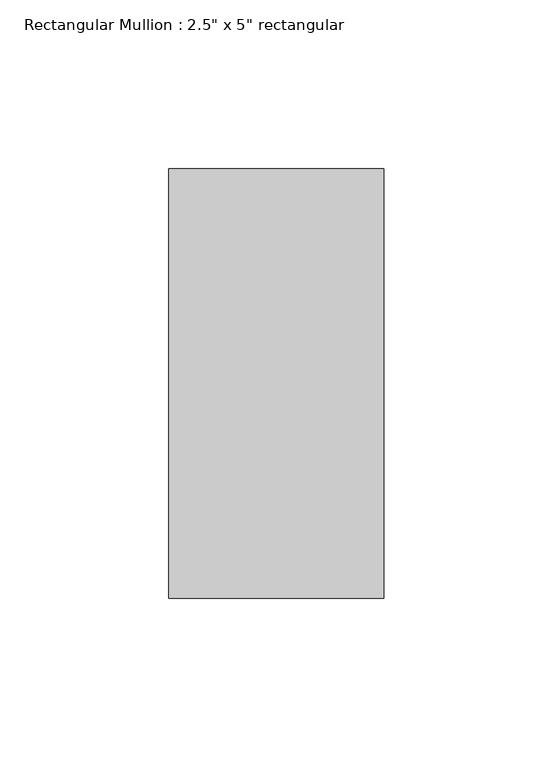
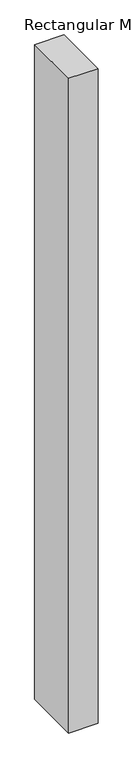
"""IFC4 building model written with IfcOpenShell, lengths in millimetres: member geometry."""

from ifc_helpers import new_model, si_unit, frame, origin, place, context, project, spatial, polyline, outline, extrude, source, transform, mapped, element, save


def member_177cc448(model_context):
    return source(origin(), model_context, "Body", "SweptSolid", [
        extrude(outline(polyline([(0.0, 63.5), (0.0, -63.5), (-63.5, -63.5), (-63.5, 63.5), (0.0, 63.5)])), frame((0.0, 0.0, -1493.5474484), z_axis=(0.0, 0.0, 1.0), x_axis=(1.0, 0.0, 0.0)), (0.0, 0.0, 1.0), 1493.5474484),
    ])


if __name__ == "__main__":
    model = new_model("IFC4")
    model_context = context("Model", 3, world=origin())
    ifc_project = project(units=[si_unit("LENGTHUNIT", "METRE", prefix="MILLI")], contexts=[model_context])
    site = spatial("IfcSite", under=ifc_project)
    building = spatial("IfcBuilding", under=site)
    placement = place(None, origin())
    member_shape = member_177cc448(model_context)
    element("IfcMember", 1, ObjectType="Rectangular Mullion : 2.5\" x 5\" rectangular", at=placement, inside=building, context=model_context, shape_type="MappedRepresentation", body=[
        mapped(member_shape, transform((0.0, 0.0, 0.0), x_axis=(1.0, 0.0, 0.0), y_axis=(0.0, 1.0, 0.0), z_axis=(0.0, 0.0, 1.0))),
    ])
    save(model, "model.ifc")

# Revit data of these elements
# Type "Rectangular Mullion : 2.5\" x 5\" rectangular"
#   built-in parameter 1007304 = 0.416667 (stored number, unit not read)
#   built-in parameter 1007301 = 0.104167 (stored number, unit not read)
#   built-in parameter 1007300 = 0.104167 (stored number, unit not read)
# Element 1 (IfcMember, "Rectangular Mullion : 2.5\" x 5\" rectangular")
#   Materials on its faces: "Aluminum"
# Materials
#   "Aluminum": class "Metal", colour RGB 247 247 247, transparency 0, Description = "Aluminum 6061", Cost = 0
